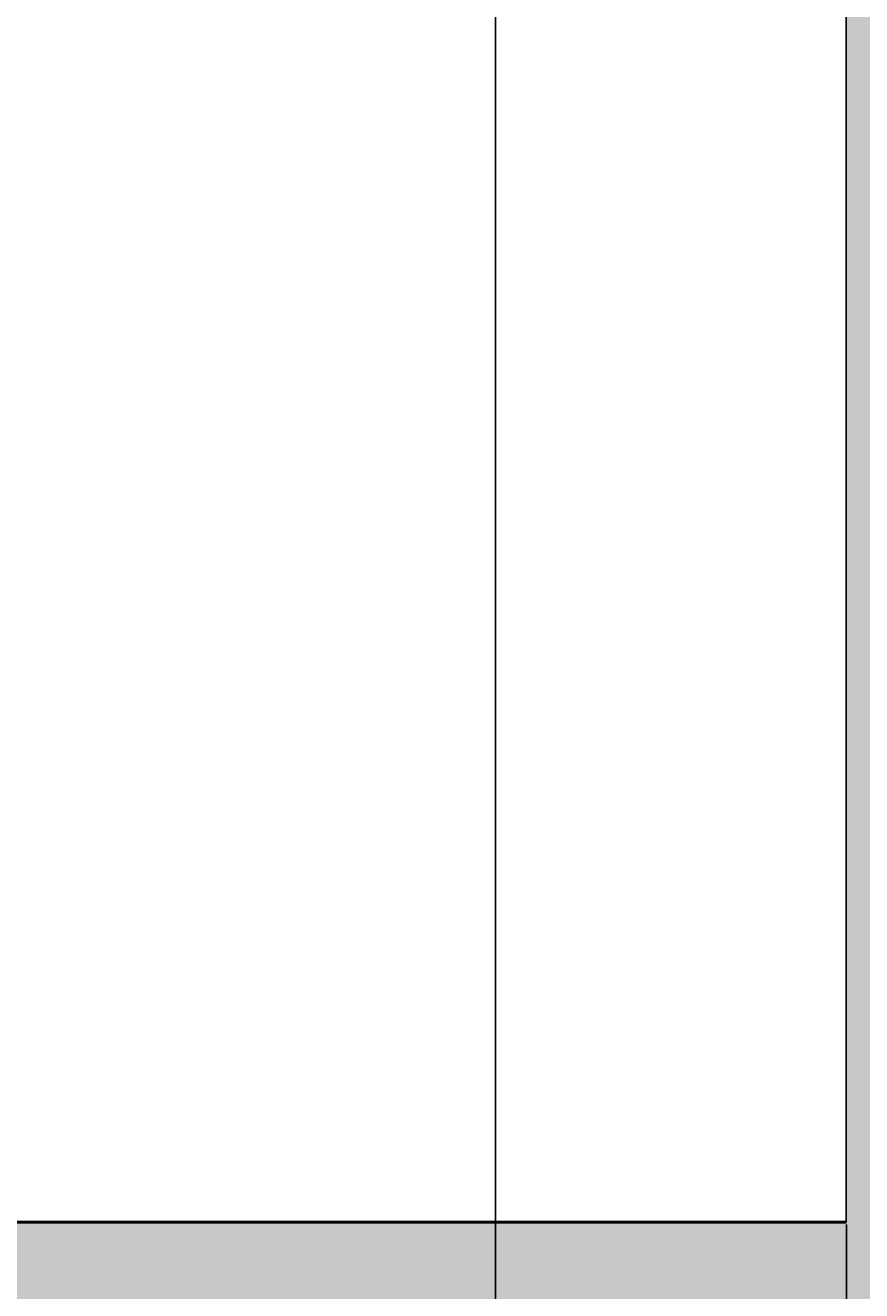
# Model space of a CAD drawing. Units: inches. Extents: x 2231 to 2461, y 2045 to 2455.
# Tile 57 of 95: x 2371 to 2395, y 2185 to 2222. Entities that reach past the tile are written whole.
import ezdxf

# ---------------------------------------------------------------- set-up
doc = ezdxf.new("R2010")
doc.units = ezdxf.units.IN
for name, color, linetype, lineweight in [('A-ANNO-DIMS', 2, 'Continuous', 18), ('A-FLOR-STRS', 7, 'Continuous', 25), ('A-WALL', 7, 'Continuous', 50)]:
    doc.layers.add(name, color=color, linetype=linetype, lineweight=lineweight)
doc.layers.add('A-WALL-PATT', color=18, linetype='Continuous', lineweight=13, true_color=0x000000)
doc.styles.get("Standard").update_dxf_attribs({"font": 'arial.ttf'})
doc.dimstyles.get("Standard").update_dxf_attribs({"dimtxt": 0.18, "dimasz": 0.18, "dimexe": 0.18, "dimexo": 0.0625, "dimgap": 0.09, "dimtad": 0, "dimtih": 1, "dimtoh": 1, "dimdec": 4, "dimzin": 0, "dimdsep": 46, "dimtxsty": 'Standard', "dimcen": 0.09, "dimadec": 0, "dimazin": 0, "dimtfac": 1, "dimtdec": 4, "dimtofl": 0, "dimtmove": 0, "dimatfit": 3, "dimfxl": 1, "dimtolj": 1, "dimtzin": 0, "dimarcsym": 0})

# ---------------------------------------------------------------- blocks, each defined once
blk = doc.blocks.new('*D66')
at = {"layer": 'A-ANNO-DIMS', "color": 0, "lineweight": -2, "transparency": 16777216}
for p, q in [((2348.189, 2096.895), (2348.189, 2454.645)), ((2408.794, 2096.895), (2408.794, 2454.645)), ((2348.369, 2454.465), (2378.167, 2454.465)), ((2408.614, 2454.465), (2378.815, 2454.465))]:
    blk.add_line(p, q, dxfattribs=at)
at = {"layer": 'A-ANNO-DIMS', "color": 0, "transparency": 16777216}
for points in [[(2348.369, 2454.495), (2348.369, 2454.435), (2348.189, 2454.465)], [(2408.614, 2454.495), (2408.614, 2454.435), (2408.794, 2454.465)]]:
    blk.add_solid(points, dxfattribs=at)
at = {"layer": 'Defpoints', "color": 0, "transparency": 16777216}
for p in [(2408.794, 2454.465), (2348.189, 2096.833), (2408.794, 2096.833)]:
    blk.add_point(p, dxfattribs=at)
at = {"layer": 'A-ANNO-DIMS', "color": 0, "transparency": 16777216, "insert": (2378.491, 2454.465), "char_height": 0.18, "attachment_point": 5}
blk.add_mtext('\\A1;60.6', dxfattribs=at)
blk = doc.blocks.new('*D69')
at = {"layer": 'A-ANNO-DIMS', "color": 0, "lineweight": -2, "transparency": 16777216}
for p, q in [((2340.667, 2189.285), (2340.667, 2044.803)), ((2394.794, 2186.77), (2394.794, 2044.803)), ((2340.847, 2044.983), (2367.337, 2044.983)), ((2394.614, 2044.983), (2368.124, 2044.983))]:
    blk.add_line(p, q, dxfattribs=at)
at = {"layer": 'A-ANNO-DIMS', "color": 0, "transparency": 16777216}
for points in [[(2340.847, 2045.013), (2340.847, 2044.953), (2340.667, 2044.983)], [(2394.614, 2045.013), (2394.614, 2044.953), (2394.794, 2044.983)]]:
    blk.add_solid(points, dxfattribs=at)
at = {"layer": 'Defpoints', "color": 0, "transparency": 16777216}
for p in [(2340.667, 2189.348), (2394.794, 2186.833), (2394.794, 2044.983)]:
    blk.add_point(p, dxfattribs=at)
at = {"layer": 'A-ANNO-DIMS', "color": 0, "transparency": 16777216, "insert": (2367.73, 2044.983), "char_height": 0.18, "attachment_point": 5}
blk.add_mtext('\\A1;54.13', dxfattribs=at)
blk = doc.blocks.new('*D72')
at = {"layer": 'A-ANNO-DIMS', "color": 0, "lineweight": -2, "transparency": 16777216}
for p, q in [((2384.543, 2145.12), (2384.543, 2454.645)), ((2408.794, 2150.677), (2408.794, 2454.645)), ((2384.723, 2454.465), (2396.272, 2454.465)), ((2408.614, 2454.465), (2397.064, 2454.465))]:
    blk.add_line(p, q, dxfattribs=at)
at = {"layer": 'A-ANNO-DIMS', "color": 0, "transparency": 16777216}
for points in [[(2384.723, 2454.495), (2384.723, 2454.435), (2384.543, 2454.465)], [(2408.614, 2454.495), (2408.614, 2454.435), (2408.794, 2454.465)]]:
    blk.add_solid(points, dxfattribs=at)
at = {"layer": 'Defpoints', "color": 0, "transparency": 16777216}
for p in [(2408.794, 2454.465), (2408.794, 2150.615), (2384.543, 2145.058)]:
    blk.add_point(p, dxfattribs=at)
at = {"layer": 'A-ANNO-DIMS', "color": 0, "transparency": 16777216, "insert": (2396.668, 2454.465), "char_height": 0.18, "attachment_point": 5}
blk.add_mtext('\\A1;24.25', dxfattribs=at)

msp = doc.modelspace()

# ---------------------------------------------------------------- hatches: boundary and pattern name
at = {"layer": 'A-WALL-PATT'}
h = msp.add_hatch(color=256, dxfattribs=at)
h.dxf.hatch_style = 1
h.paths.add_polyline_path([(2441.7935, 2269.1535), (2432.7935, 2269.1535), (2432.7935, 2186.8328), (2396.7935, 2186.8328), (2396.7935, 2286.8328), (2394.7935, 2286.8328), (2394.7935, 2186.8328), (2334.7935, 2186.8328), (2334.7935, 2182.8328), (2432.7935, 2182.8328), (2432.7935, 2072.8328), (2416.6639, 2072.8328), (2416.6639, 2063.8328), (2441.7935, 2063.8328)])
h.paths.add_polyline_path([(2368.6639, 2072.8328), (2367.04, 2072.8328), (2330.7942, 2072.8328), (2330.7397, 2063.8328), (2368.6639, 2063.8328)])
h.paths.add_polyline_path([(2300.7392, 2068.3328), (2300.7392, 2072.8328), (2298.7935, 2072.8328), (2294.7935, 2072.8328), (2258.7935, 2072.8328), (2258.7935, 2120.8328), (2294.7935, 2120.8328), (2298.7935, 2120.8328), (2298.7935, 2128.8328), (2294.7935, 2128.8328), (2294.7935, 2124.8328), (2258.7935, 2124.8328), (2258.7935, 2182.8328), (2294.7935, 2182.8328), (2294.7935, 2174.8328), (2298.7935, 2174.8328), (2298.7935, 2182.8328), (2304.7935, 2182.8328), (2304.7935, 2186.8328), (2258.7935, 2186.8328), (2258.7935, 2221.999), (2249.7935, 2221.999), (2249.7935, 2063.8328), (2300.7392, 2063.8328)])
h.paths.add_polyline_path([(2391.9338, 2435.8328), (2333.82, 2435.8328), (2333.82, 2426.8328), (2368.7935, 2426.8328), (2368.7935, 2374.9508), (2368.7935, 2370.8328), (2372.3935, 2370.8328), (2372.7935, 2370.8328), (2372.7935, 2426.8328), (2391.9338, 2426.8328)])
h.paths.add_polyline_path([(2441.7935, 2435.8328), (2415.9338, 2435.8328), (2415.9338, 2426.8328), (2432.7935, 2426.8328), (2432.7935, 2334.8328), (2372.7935, 2334.8328), (2372.7935, 2346.8328), (2368.7935, 2346.8328), (2368.7935, 2306.8328), (2360.7935, 2306.8328), (2360.7935, 2302.8328), (2368.7935, 2302.8328), (2372.7935, 2302.8328), (2372.7935, 2330.8328), (2432.7935, 2330.8328), (2432.7935, 2317.1535), (2441.7935, 2317.1535)])
h.paths.add_polyline_path([(2285.82, 2435.8328), (2249.7935, 2435.8328), (2249.7935, 2269.999), (2258.7935, 2269.999), (2258.7935, 2302.8328), (2318.8168, 2302.8328), (2330.7935, 2302.8328), (2330.7935, 2306.8328), (2258.7935, 2306.8328), (2258.7935, 2426.8328), (2285.82, 2426.8328)])

# ---------------------------------------------------------------- linework, layer by layer
at = {"layer": 'A-FLOR-STRS'}
msp.add_line((2394.7935, 2286.8328), (2394.7935, 2186.8328), dxfattribs=at)
at = {"layer": 'A-WALL'}
msp.add_line((2334.7935, 2186.8328), (2394.7935, 2186.8328), dxfattribs=at)

# ---------------------------------------------------------------- dimensions: what is measured, and where the dimension line sits
at = {"layer": 'A-ANNO-DIMS'}
for base, p1, p2, override, picture, middle in [((2408.7935, 2454.4653), (2348.1888, 2096.8328), (2408.7935, 2096.8328), {"dimdec": 1, "dimlfac": 1, "dimrnd": 0, "dimzin": 0, "dimdsep": 46, "dimlunit": 2}, '*D66', (2378.4912, 2454.4653)), ((2408.7935, 2454.4653), (2384.5428, 2145.0576), (2408.7935, 2150.6145), {"dimdec": 2, "dimlfac": 1, "dimrnd": 0, "dimzin": 0, "dimdsep": 46, "dimlunit": 2}, '*D72', (2396.6682, 2454.4653)), ((2394.7935, 2044.9825), (2340.6673, 2189.3477), (2394.7935, 2186.8328), {"dimdec": 2, "dimlfac": 1, "dimrnd": 0, "dimzin": 0, "dimdsep": 46, "dimlunit": 2}, '*D69', (2367.7304, 2044.9825))]:
    dim = msp.add_linear_dim(base=base, p1=p1, p2=p2, dimstyle='Standard', override=override, dxfattribs=at)
    dim.commit()
    dim.dimension.update_dxf_attribs({"geometry": picture, "text_midpoint": middle})

doc.saveas('drawing.dxf')
